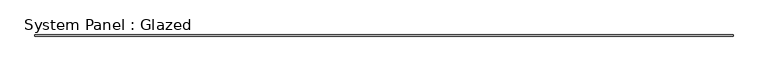
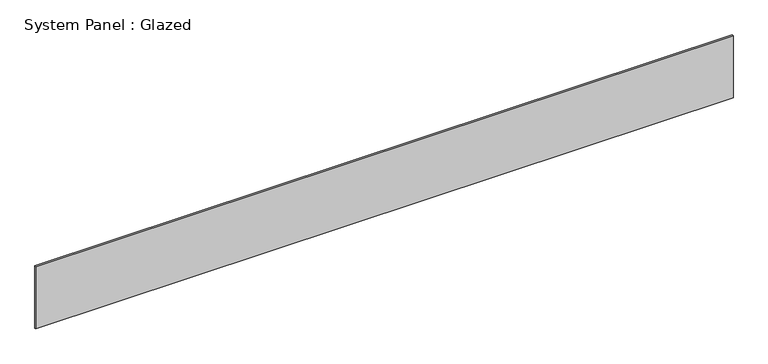
"""IFC4 building model written with IfcOpenShell, lengths in millimetres: plate geometry, System Panel : Glazed."""

from ifc_helpers import new_model, si_unit, origin, origin_with_axes, place, context, project, spatial, polyline, outline, extrude, source, transform, mapped, element, save


def system_panel_glazed_19389588(model_context):
    return source(origin(), model_context, "Body", "SweptSolid", [
        extrude(outline(polyline([(8074.025, 19.05), (-8074.025, 19.05), (-8074.025, 44.45), (8074.025, 44.45), (8074.025, 19.05)])), origin_with_axes(), (0.0, 0.0, 1.0), 1524.0),
    ])


if __name__ == "__main__":
    model = new_model("IFC4")
    model_context = context("Model", 3, world=origin())
    ifc_project = project(units=[si_unit("LENGTHUNIT", "METRE", prefix="MILLI")], contexts=[model_context])
    site = spatial("IfcSite", under=ifc_project)
    building = spatial("IfcBuilding", under=site)
    placement = place(None, origin())
    system_panel_glazed_shape = system_panel_glazed_19389588(model_context)
    element("IfcPlate", 1, ObjectType="System Panel : Glazed", at=placement, inside=building, context=model_context, shape_type="MappedRepresentation", body=[
        mapped(system_panel_glazed_shape, transform((0.0, 0.0, 0.0), x_axis=(1.0, 0.0, 0.0), y_axis=(0.0, 1.0, 0.0), z_axis=(0.0, 0.0, 1.0))),
    ])
    save(model, "model.ifc")

# Revit data of these elements
# Type "System Panel : Glazed"
#   Construction Type Id = "GSP4R"
#   Analytic Construction = "1/8 in Pilkington single glazing"
#   Visual Light Transmittance = 0.9
#   Solar Heat Gain Coefficient = 0.86
#   Heat Transfer Coefficient (U) = 1.18115 BTU/(h·ft²·°F)
# Element 1 (IfcPlate, "System Panel : Glazed")
#   Materials on its faces: "Glass"
# Materials
#   "Glass": class "Glass", colour RGB 0 128 192, transparency 0.75, Description = "Soda Lime Glass", Cost = 0
